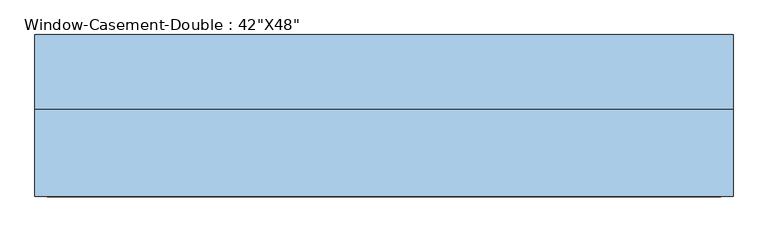
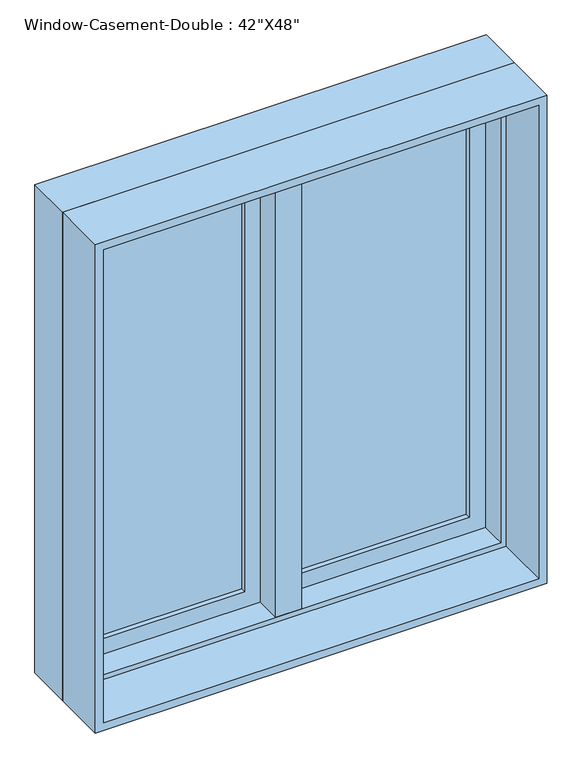
"""IFC4 building model written with IfcOpenShell, lengths in millimetres: window geometry."""

from ifc_helpers import new_model, si_unit, frame, origin, place, context, project, spatial, polyline, outline, extrude, faceted_brep, source, transform, mapped, element, save


def window_2032b2cd(model_context):
    return source(origin(), model_context, "Body", "SolidModel", [
        faceted_brep([(9.525, 133.35, 2120.9), (-9.525, 133.35, 2120.9), (-9.525, 82.55, 2120.9), (9.525, 82.55, 2120.9), (9.525, 133.35, 927.1), (9.525, 82.55, 927.1), (-9.525, 82.55, 927.1), (-9.525, 133.35, 927.1), (-9.525, 82.55, 946.15), (-9.525, 82.55, 2101.85), (-30.1625, 82.55, 946.15), (-30.1625, 82.55, 2101.85), (-30.1625, 19.05, 946.15), (-30.1625, 19.05, 2101.85), (30.1625, 19.05, 946.15), (30.1625, 19.05, 2101.85), (30.1625, 82.55, 946.15), (30.1625, 82.55, 2101.85), (9.525, 82.55, 946.15), (9.525, 82.55, 2101.85)], [[[0, 1, 2, 3]], [[4, 5, 6, 7]], [[1, 0, 4, 7]], [[2, 1, 7, 6, 8, 9]], [[9, 8, 10, 11]], [[11, 10, 12, 13]], [[13, 12, 14, 15]], [[15, 14, 16, 17]], [[17, 16, 18, 19]], [[0, 3, 19, 18, 5, 4]], [[18, 8, 6, 5]], [[9, 19, 3, 2]], [[8, 18, 16, 14, 12, 10]], [[19, 9, 11, 13, 15, 17]]]),
        extrude(outline(polyline([(-66.675, 114.3), (-66.675, 107.95), (-463.55, 107.95), (-463.55, 114.3), (-66.675, 114.3)])), frame((0.0, 0.0, 984.25), z_axis=(0.0, 0.0, 1.0), x_axis=(1.0, 0.0, 0.0)), (0.0, 0.0, 1.0), 1079.5),
        extrude(outline(polyline([(-463.55, 95.25), (-463.55, 101.6), (-66.675, 101.6), (-66.675, 95.25), (-463.55, 95.25)])), frame((0.0, 0.0, 984.25), z_axis=(0.0, 0.0, 1.0), x_axis=(1.0, 0.0, 0.0)), (0.0, 0.0, 1.0), 1079.5),
        extrude(outline(polyline([(463.55, 114.3), (463.55, 107.95), (66.675, 107.95), (66.675, 114.3), (463.55, 114.3)])), frame((0.0, 0.0, 984.25), z_axis=(0.0, 0.0, 1.0), x_axis=(1.0, 0.0, 0.0)), (0.0, 0.0, 1.0), 1079.5),
        extrude(outline(polyline([(66.675, 95.25), (66.675, 101.6), (463.55, 101.6), (463.55, 95.25), (66.675, 95.25)])), frame((0.0, 0.0, 984.25), z_axis=(0.0, 0.0, 1.0), x_axis=(1.0, 0.0, 0.0)), (0.0, 0.0, 1.0), 1079.5),
        extrude(outline(polyline([(2120.9, -520.7), (927.1, -520.7), (927.1, -9.525), (2120.9, -9.525), (2120.9, -520.7)]), holes=[polyline([(2063.75, -66.675), (984.25, -66.675), (984.25, -463.55), (2063.75, -463.55), (2063.75, -66.675)])]), frame((0.0, 82.55, 0.0), z_axis=(0.0, 1.0, 0.0), x_axis=(0.0, 0.0, 1.0)), (0.0, 0.0, 1.0), 44.45),
        extrude(outline(polyline([(927.1, 520.7), (2120.9, 520.7), (2120.9, 9.525), (927.1, 9.525), (927.1, 520.7)]), holes=[polyline([(984.25, 66.675), (2063.75, 66.675), (2063.75, 463.55), (984.25, 463.55), (984.25, 66.675)])]), frame((0.0, 82.55, 0.0), z_axis=(0.0, 1.0, 0.0), x_axis=(0.0, 0.0, 1.0)), (0.0, 0.0, 1.0), 44.45),
        extrude(outline(polyline([(2133.6, -533.4), (914.4, -533.4), (914.4, 533.4), (2133.6, 533.4), (2133.6, -533.4)]), holes=[polyline([(2114.55, 514.35), (933.45, 514.35), (933.45, -514.35), (2114.55, -514.35), (2114.55, 514.35)])]), frame((0.0, -114.3, 0.0), z_axis=(0.0, 1.0, 0.0), x_axis=(0.0, 0.0, 1.0)), (0.0, 0.0, 1.0), 133.35),
        faceted_brep([(501.65, 82.55, 2101.85), (501.65, 19.05, 2101.85), (-501.65, 19.05, 2101.85), (-501.65, 82.55, 2101.85), (520.7, 133.35, 2120.9), (520.7, 82.55, 2120.9), (-520.7, 82.55, 2120.9), (-520.7, 133.35, 2120.9), (533.4, 19.05, 2133.6), (533.4, 133.35, 2133.6), (-533.4, 133.35, 2133.6), (-533.4, 19.05, 2133.6), (-501.65, 19.05, 946.15), (-501.65, 82.55, 946.15), (-520.7, 82.55, 927.1), (-520.7, 133.35, 927.1), (-533.4, 133.35, 914.4), (-533.4, 19.05, 914.4), (501.65, 19.05, 946.15), (501.65, 82.55, 946.15), (520.7, 82.55, 927.1), (520.7, 133.35, 927.1), (533.4, 133.35, 914.4), (533.4, 19.05, 914.4)], [[[0, 1, 2, 3]], [[4, 5, 6, 7]], [[8, 9, 10, 11]], [[3, 2, 12, 13]], [[7, 6, 14, 15]], [[11, 10, 16, 17]], [[13, 12, 18, 19]], [[15, 14, 20, 21]], [[17, 16, 22, 23]], [[11, 17, 23, 8], [1, 18, 12, 2]], [[19, 18, 1, 0]], [[5, 20, 14, 6], [3, 13, 19, 0]], [[21, 20, 5, 4]], [[23, 22, 9, 8]], [[9, 22, 16, 10], [7, 15, 21, 4]]]),
    ])


if __name__ == "__main__":
    model = new_model("IFC4")
    model_context = context("Model", 3, world=origin())
    ifc_project = project(units=[si_unit("LENGTHUNIT", "METRE", prefix="MILLI")], contexts=[model_context])
    site = spatial("IfcSite", under=ifc_project)
    building = spatial("IfcBuilding", under=site)
    placement = place(None, origin())
    window_shape = window_2032b2cd(model_context)
    element("IfcWindow", 1, ObjectType="Window-Casement-Double : 42\"X48\"", at=placement, inside=building, context=model_context, shape_type="MappedRepresentation", body=[
        mapped(window_shape, transform((0.0, 0.0, 0.0), x_axis=(1.0, 0.0, 0.0), y_axis=(0.0, 1.0, 0.0), z_axis=(0.0, 0.0, 1.0))),
    ])
    save(model, "model.ifc")

# Revit data of these elements
# Type "Window-Casement-Double : 42\"X48\""
#   Type Mark = "27"
#   Fire Rating = "0.5h"
#   Assembly Code = "B2020100"
#   Analytic Construction = "Double glazing - domestic"
#   Frame Extension [instance default] = 0' - 0 1/4"
#   Window Inset [instance default] = 0' - 0"
#   Wall Thickness [instance default] = 0' - 6"
#   Interior Wall Closure [instance default] = 0' - 2 1/4"
#   Half Width = 1' - 9"
#   Visual Light Transmittance = 0.81
#   Thermal Resistance (R) = 1.8146 (h·ft²·°F)/BTU
#   Solar Heat Gain Coefficient = 0.76
#   Rough Width = 3' - 6 1/2"
#   Rough Height = 4' - 0 1/2"
#   Height = 4' - 0"
#   Heat Transfer Coefficient (U) = 0.5511 BTU/(h·ft²·°F)
#   Exterior Wall Closure [instance default] = 0' - 1 1/4"
#   Extension Jamb [instance default] = 0' - 2 1/4"
#   Default Sill Height = 3' - 0"
#   Width = 3' - 6"
#   Muntin Visibility = yes
#   Interior Trim Visibility [instance default] = yes
#   Exterior Trim Visibility [instance default] = yes
#   Extension Jamb Visibility [instance default] = yes
#   Interior Trim Material = Wood - Stained
#   Muntin Pattern = Muntin Pattern_2x2 : Muntin Pattern_2x2
#   Interior Trim = Trim-Window-Interior-Flat : Picture Frame
#   Interior Frame Material = Wood - Stained
#   Glass Panel Material = Glass
#   Exterior Trim Material = Clad - White
#   Exterior Trim = Trim-Window-Exterior-Flat : with Sill
#   Exterior Frame Material = Clad - White
#   Wall Closure = (empty or 0)
# Element 1 (IfcWindow, "Window-Casement-Double : 42\"X48\"")
#   Wall Thickness = 0' - 9"
#   Extension Jamb = 0' - 5 1/4"
#   Materials on its faces: "Wood - Stained", "Glass", "Clad - White"
# Materials
#   "Wood - Stained": class "Wood", colour RGB 224 178 126, transparency 0, Cost = 0
#   "Glass": class "Glass", colour RGB 0 128 192, transparency 0.75, Description = "Soda Lime Glass", Cost = 0
#   "Clad - White": class "Wood", colour RGB 242 242 238, transparency 0, Cost = 0
